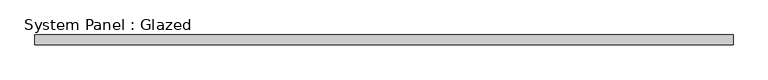
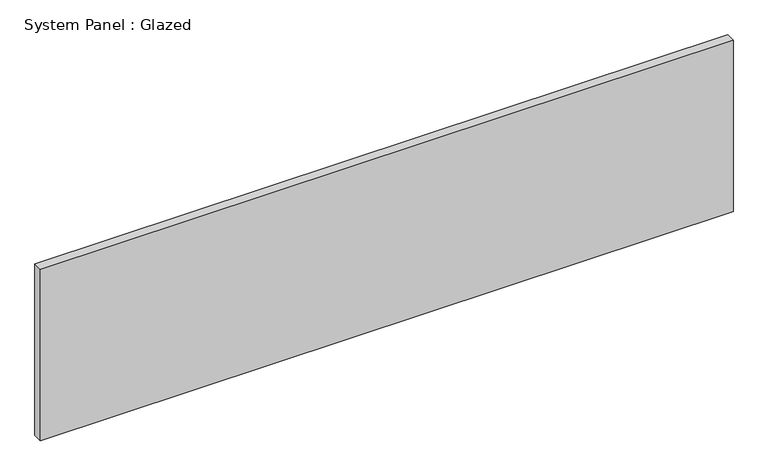
"""IFC4 building model written with IfcOpenShell, lengths in millimetres: plate geometry, System Panel : Glazed."""

from ifc_helpers import new_model, si_unit, origin, origin_with_axes, place, context, project, spatial, polyline, outline, extrude, source, transform, mapped, element, save


def system_panel_glazed_3dd2ea40(model_context):
    return source(origin(), model_context, "Body", "SweptSolid", [
        extrude(outline(polyline([(917.575, 19.05), (-917.575, 19.05), (-917.575, 44.45), (917.575, 44.45), (917.575, 19.05)])), origin_with_axes(), (0.0, 0.0, 1.0), 480.6386718),
    ])


if __name__ == "__main__":
    model = new_model("IFC4")
    model_context = context("Model", 3, world=origin())
    ifc_project = project(units=[si_unit("LENGTHUNIT", "METRE", prefix="MILLI")], contexts=[model_context])
    site = spatial("IfcSite", under=ifc_project)
    building = spatial("IfcBuilding", under=site)
    placement = place(None, origin())
    system_panel_glazed_shape = system_panel_glazed_3dd2ea40(model_context)
    element("IfcPlate", 1, ObjectType="System Panel : Glazed", at=placement, inside=building, context=model_context, shape_type="MappedRepresentation", body=[
        mapped(system_panel_glazed_shape, transform((0.0, 0.0, 0.0), x_axis=(1.0, 0.0, 0.0), y_axis=(0.0, 1.0, 0.0), z_axis=(0.0, 0.0, 1.0))),
    ])
    save(model, "model.ifc")

# Revit data of these elements
# Type "System Panel : Glazed"
#   Construction Type Id = "GSP4R"
#   Analytic Construction = "1/8 in Pilkington single glazing"
#   Visual Light Transmittance = 0.9
#   Solar Heat Gain Coefficient = 0.86
#   Heat Transfer Coefficient (U) = 1.18115 BTU/(h·ft²·°F)
#   Define Thermal Properties by = 1
# Element 1 (IfcPlate, "System Panel : Glazed")
#   Materials on its faces: "Glass"
# Materials
#   "Glass": class "Glass", colour RGB 0 128 192, transparency 0.75, Description = "Soda Lime Glass", Cost = 0
